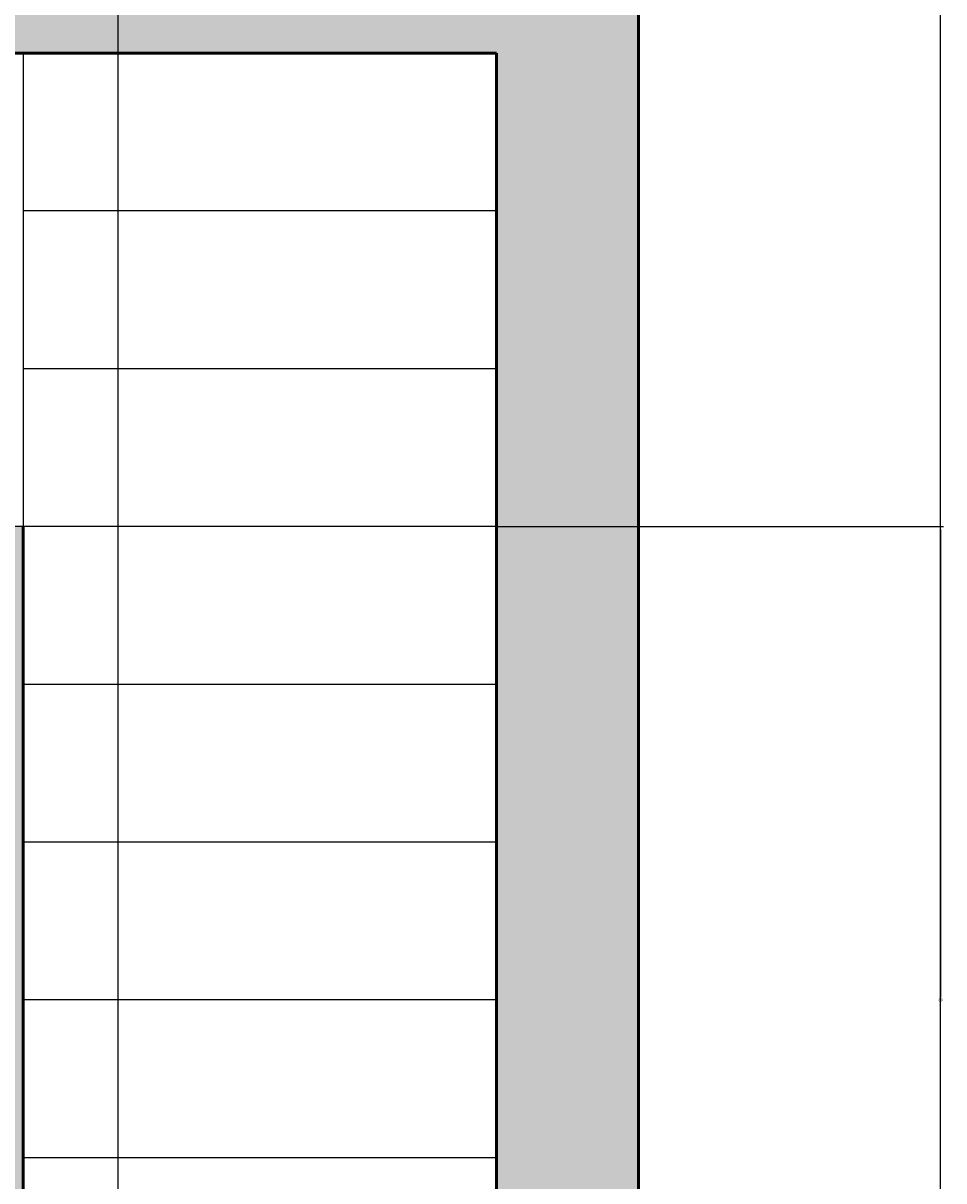
# Model space of a CAD drawing. Units: inches. Extents: x 2307 to 2544, y 2171 to 2540.
# Tile 14 of 52: x 2486 to 2544, y 2244 to 2317. Entities that reach past the tile are written whole.
import ezdxf

# ---------------------------------------------------------------- set-up
doc = ezdxf.new("R2010")
doc.units = ezdxf.units.IN
for name, color, linetype, lineweight in [('A-ANNO-DIMS', 2, 'Continuous', 18), ('A-FLOR-STRS', 7, 'Continuous', 25), ('A-WALL', 7, 'Continuous', 50)]:
    doc.layers.add(name, color=color, linetype=linetype, lineweight=lineweight)
doc.layers.add('A-WALL-PATT', color=18, linetype='Continuous', lineweight=13, true_color=0x000000)
doc.styles.get("Standard").update_dxf_attribs({"font": 'arial.ttf'})
doc.dimstyles.get("Standard").update_dxf_attribs({"dimtxt": 0.18, "dimasz": 0.18, "dimexe": 0.18, "dimexo": 0.0625, "dimgap": 0.09, "dimtad": 0, "dimtih": 1, "dimtoh": 1, "dimdec": 4, "dimzin": 0, "dimdsep": 46, "dimtxsty": 'Standard', "dimcen": 0.09, "dimadec": 0, "dimazin": 0, "dimtfac": 1, "dimtdec": 4, "dimtofl": 0, "dimtmove": 0, "dimatfit": 3, "dimfxl": 1, "dimtolj": 1, "dimtzin": 0, "dimarcsym": 0})

# ---------------------------------------------------------------- blocks, each defined once
blk = doc.blocks.new('*D37')
at = {"layer": 'A-ANNO-DIMS', "color": 0, "lineweight": -2, "transparency": 16777216}
for p, q in [((2524.758, 2520.51), (2544.026, 2520.51)), ((2543.846, 2520.33), (2543.846, 2355.692)), ((2543.846, 2190.69), (2543.846, 2355.328)), ((2524.758, 2190.51), (2544.026, 2190.51))]:
    blk.add_line(p, q, dxfattribs=at)
at = {"layer": 'A-ANNO-DIMS', "color": 0, "transparency": 16777216}
for points in [[(2543.816, 2520.33), (2543.876, 2520.33), (2543.846, 2520.51)], [(2543.816, 2190.69), (2543.876, 2190.69), (2543.846, 2190.51)]]:
    blk.add_solid(points, dxfattribs=at)
at = {"layer": 'Defpoints', "color": 0, "transparency": 16777216}
for p in [(2524.696, 2520.51), (2543.846, 2520.51), (2524.696, 2190.51)]:
    blk.add_point(p, dxfattribs=at)
at = {"layer": 'A-ANNO-DIMS', "color": 0, "transparency": 16777216, "insert": (2543.846, 2355.51), "char_height": 0.18, "attachment_point": 5}
blk.add_mtext('\\A1;330', dxfattribs=at)
blk = doc.blocks.new('*D54')
at = {"layer": 'A-ANNO-DIMS', "color": 0, "lineweight": -2, "transparency": 16777216}
for p, q in [((2461.696, 2435.447), (2461.696, 2171.18)), ((2491.696, 2435.447), (2491.696, 2171.18)), ((2461.876, 2171.36), (2476.477, 2171.36)), ((2491.516, 2171.36), (2476.914, 2171.36))]:
    blk.add_line(p, q, dxfattribs=at)
at = {"layer": 'A-ANNO-DIMS', "color": 0, "transparency": 16777216}
for points in [[(2461.876, 2171.39), (2461.876, 2171.33), (2461.696, 2171.36)], [(2491.516, 2171.39), (2491.516, 2171.33), (2491.696, 2171.36)]]:
    blk.add_solid(points, dxfattribs=at)
at = {"layer": 'Defpoints', "color": 0, "transparency": 16777216}
for p in [(2461.696, 2435.51), (2491.696, 2435.51), (2491.696, 2171.36)]:
    blk.add_point(p, dxfattribs=at)
at = {"layer": 'A-ANNO-DIMS', "color": 0, "transparency": 16777216, "insert": (2476.696, 2171.36), "char_height": 0.18, "attachment_point": 5}
blk.add_mtext('\\A1;30', dxfattribs=at)
blk = doc.blocks.new('*D56')
at = {"layer": 'A-ANNO-DIMS', "color": 0, "lineweight": -2, "transparency": 16777216}
for p, q in [((2515.758, 2285.51), (2544.026, 2285.51)), ((2543.846, 2285.33), (2543.846, 2255.691)), ((2543.846, 2225.69), (2543.846, 2255.328)), ((2515.758, 2225.51), (2544.026, 2225.51))]:
    blk.add_line(p, q, dxfattribs=at)
at = {"layer": 'A-ANNO-DIMS', "color": 0, "transparency": 16777216}
for points in [[(2543.816, 2285.33), (2543.876, 2285.33), (2543.846, 2285.51)], [(2543.816, 2225.69), (2543.876, 2225.69), (2543.846, 2225.51)]]:
    blk.add_solid(points, dxfattribs=at)
at = {"layer": 'Defpoints', "color": 0, "transparency": 16777216}
for p in [(2515.696, 2285.51), (2543.846, 2285.51), (2515.696, 2225.51)]:
    blk.add_point(p, dxfattribs=at)
at = {"layer": 'A-ANNO-DIMS', "color": 0, "transparency": 16777216, "insert": (2543.846, 2255.51), "char_height": 0.18, "attachment_point": 5}
blk.add_mtext('\\A1;60', dxfattribs=at)

msp = doc.modelspace()

# ---------------------------------------------------------------- hatches: boundary and pattern name
at = {"layer": 'A-WALL-PATT'}
h = msp.add_hatch(color=256, dxfattribs=at)
h.dxf.hatch_style = 1
h.paths.add_polyline_path([(2433.6935, 2199.5096), (2415.6423, 2199.5096), (2415.6423, 2190.5096), (2433.7832, 2190.5096)], flags=17)
h.paths.add_polyline_path([(2367.6423, 2199.5096), (2335.6958, 2199.5096), (2335.6958, 2307.3983), (2326.6958, 2307.3983), (2326.6958, 2190.5096), (2367.6423, 2190.5096)])
h.paths.add_polyline_path([(2524.6958, 2520.5096), (2496.7832, 2520.5096), (2496.7832, 2515.5149), (2472.7832, 2515.5149), (2472.7832, 2520.5096), (2415.4028, 2520.5096), (2415.4028, 2511.5096), (2451.6958, 2511.5096), (2451.6958, 2439.5096), (2451.6958, 2391.5096), (2445.6958, 2391.5096), (2445.6958, 2387.5096), (2455.6958, 2387.5096), (2455.6958, 2435.5096), (2461.6958, 2435.5096), (2461.6958, 2439.5096), (2455.6958, 2439.5096), (2455.6958, 2511.5096), (2515.6958, 2511.5096), (2515.6958, 2439.5096), (2491.6958, 2439.5096), (2491.6958, 2435.5096), (2515.6958, 2435.5096), (2515.6958, 2319.5096), (2451.6958, 2319.5096), (2451.6958, 2281.5096), (2481.6958, 2281.5096), (2481.6958, 2225.5096), (2485.6958, 2225.5096), (2485.6958, 2285.5096), (2455.6958, 2285.5096), (2455.6958, 2315.5096), (2515.6958, 2315.5096), (2515.6958, 2199.5096), (2469.6952, 2199.5096), (2469.785, 2190.5096), (2524.6958, 2190.5096)])

# ---------------------------------------------------------------- linework, layer by layer
at = {"layer": 'A-FLOR-STRS'}
for p, q in [((2485.6958, 2315.5096), (2485.6958, 2285.5096)), ((2515.6958, 2305.5096), (2485.6958, 2305.5096)), ((2515.6958, 2295.5096), (2485.6958, 2295.5096)), ((2515.6958, 2285.5096), (2455.6958, 2285.5096)), ((2515.6958, 2275.5096), (2485.6958, 2275.5096)), ((2515.6958, 2265.5096), (2485.6958, 2265.5096)), ((2515.6958, 2255.5096), (2485.6958, 2255.5096)), ((2515.6958, 2245.5096), (2485.6958, 2245.5096))]:
    msp.add_line(p, q, dxfattribs=at)
at = {"layer": 'A-WALL'}
for p, q in [((2515.6958, 2315.5096), (2455.6958, 2315.5096)), ((2515.6958, 2315.5096), (2515.6958, 2199.5096)), ((2485.6958, 2285.5096), (2485.6958, 2225.5096))]:
    msp.add_line(p, q, dxfattribs=at)
msp.add_lwpolyline([(2433.7832, 2190.5096), (2326.6958, 2190.5096), (2326.6958, 2520.5096), (2524.6958, 2520.5096), (2524.6958, 2190.5096), (2469.785, 2190.5096)], dxfattribs=at)

# ---------------------------------------------------------------- dimensions: what is measured, and where the dimension line sits
at = {"layer": 'A-ANNO-DIMS'}
for base, p1, p2, picture, middle in [((2543.8458, 2520.5096), (2524.6958, 2190.5096), (2524.6958, 2520.5096), '*D37', (2543.8458, 2355.5096)), ((2543.8458, 2285.5096), (2515.6958, 2225.5096), (2515.6958, 2285.5096), '*D56', (2543.8458, 2255.5096))]:
    dim = msp.add_linear_dim(base=base, p1=p1, p2=p2, angle=90, dimstyle='Standard', override={"dimdec": 0, "dimlfac": 1, "dimrnd": 0, "dimzin": 0, "dimdsep": 46, "dimlunit": 2}, dxfattribs=at)
    dim.commit()
    dim.dimension.update_dxf_attribs({"geometry": picture, "text_midpoint": middle})
dim = msp.add_linear_dim(base=(2491.6958, 2171.3596), p1=(2461.6958, 2435.5096), p2=(2491.6958, 2435.5096), dimstyle='Standard', override={"dimdec": 0, "dimlfac": 1, "dimrnd": 0, "dimzin": 0, "dimdsep": 46, "dimlunit": 2}, dxfattribs=at)
dim.commit()
dim.dimension.update_dxf_attribs({"geometry": '*D54', "text_midpoint": (2476.6958, 2171.3596)})

doc.saveas('drawing.dxf')
